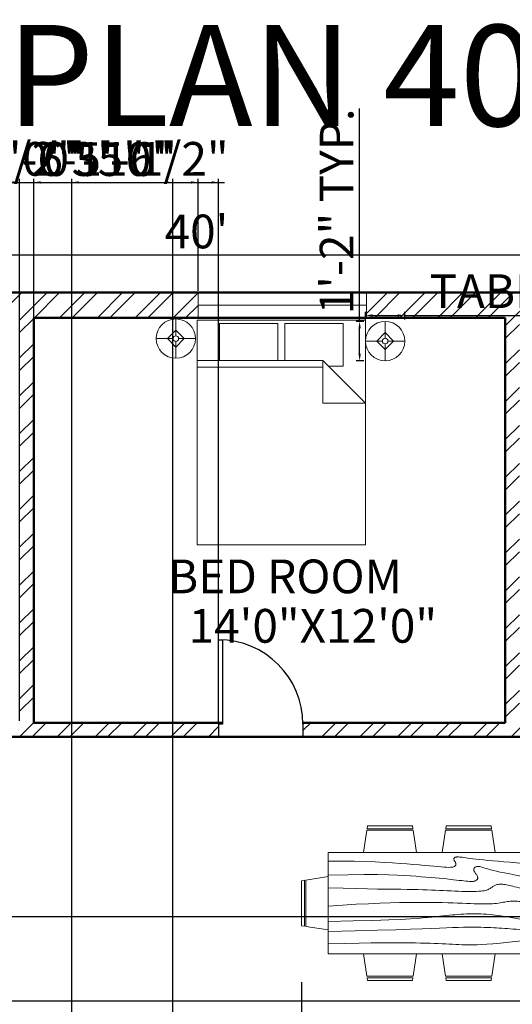
# Model space of a CAD drawing. Units: inches. Extents: x 1954 to 2815, y 1733 to 2371.
# Tile 3 of 4: x 2417 to 2592, y 2012 to 2362. Entities that reach past the tile are written whole.
import ezdxf

# ---------------------------------------------------------------- set-up
doc = ezdxf.new("R2010")
doc.units = ezdxf.units.IN
for name, color, linetype, lineweight in [('A-ANNO-DIMS', 2, 'Continuous', 18), ('A-ANNO-TEXT', 7, 'Continuous', 25), ('A-AREA-IDEN', 7, 'Continuous', 25), ('A-DOOR', 3, 'Continuous', 25), ('A-FURN', 8, 'Continuous', 18), ('A-GLAZ', 4, 'Continuous', 18), ('A-WALL', 7, 'Continuous', 50), ('A-WALL-PATT', 252, 'Continuous', 13)]:
    doc.layers.add(name, color=color, linetype=linetype, lineweight=lineweight)
doc.styles.get("Standard").update_dxf_attribs({"font": 'arial.ttf'})
doc.dimstyles.new('ISO-25', dxfattribs={"dimtxt": 12, "dimasz": 2.5, "dimexe": 1.25, "dimexo": 0.625, "dimtad": 1, "dimdec": 1, "dimlunit": 4, "dimtxsty": 'Standard', "dimcen": 2.5, "dimadec": 0, "dimazin": 0, "dimtfac": 1, "dimtdec": 1, "dimtmove": 0, "dimatfit": 3, "dimfxl": 1, "dimarcsym": 0})

# ---------------------------------------------------------------- blocks, each defined once
blk = doc.blocks.new('*U2')
for p, q in [((0, 0), (0, -6)), ((40, 0), (40, -6))]:
    blk.add_line(p, q)
blk.add_lwpolyline([(0, 0), (0, 40), (1.75, 40), (1.75, 0)], close=True)
blk.add_arc((0, 0), 40, 0, 90)
blk = doc.blocks.new('Bed - Queen')
for p, q in [((0, -80.00003), (0, 0)), ((0, 0), (59.99999, 0)), ((59.99999, 0), (59.99999, -80.00003)), ((7.99999, -1.2), (28.79998, -1.2)), ((7.99999, -14.4), (7.99999, -1.2)), ((28.79998, -1.2), (28.79998, -14.4)), ((31.19999, -1.2), (51.99999, -1.2)), ((31.19999, -14.4), (31.19999, -1.2)), ((51.99999, -1.2), (51.99999, -16.4)), ((0, -14.4), (44.8, -14.4)), ((44.8, -16.8), (0, -16.8)), ((59.99999, -29.6), (44.8, -14.4)), ((44.8, -14.4), (44.8, -29.6)), ((51.99999, -16.4), (46.79936, -16.4)), ((44.8, -29.6), (59.99999, -29.6)), ((59.99999, -80.00003), (0, -80.00003))]:
    blk.add_line(p, q)
blk = doc.blocks.new('Lamp - Table')
for p, q in [((0, 7), (0, 1)), ((-1, 0), (-7, 0)), ((0, 3), (-3, 0)), ((-3, 0), (0, -3)), ((3, 0), (0, 3)), ((0, -3), (3, 0)), ((1, 0), (7, 0)), ((0, -1), (0, -7))]:
    blk.add_line(p, q)
for radius in [7, 1]:
    blk.add_circle((0, 0), radius)
blk = doc.blocks.new('Dining Set - 36 x 72 in.')
for p, q in [((-22.2343, 26.00059), (-23.4847, 17.99762)), ((-22.2304, 26), (-5.7608, 26)), ((-22, 27.5), (-22.1562, 26.50042)), ((-5.8416, 26.5), (-22.1534, 26.5)), ((-22, 27.5), (-6, 27.5)), ((-5.8437, 26.49966), (-6, 27.5)), ((-4.5152, 17.99762), (-5.7655, 25.99926)), ((5.7657, 26.00059), (4.5153, 17.99762)), ((5.7696, 26), (22.2392, 26)), ((6, 27.5), (5.8438, 26.50042)), ((22.1584, 26.5), (5.8466, 26.5)), ((6, 27.5), (22, 27.5)), ((22.1563, 26.49966), (22, 27.5)), ((23.4848, 17.99762), (22.2345, 25.99926)), ((36, 18), (-36, 18)), ((-36, 18), (-36, -18)), ((36, -18), (36, 18)), ((-45.5, 8), (-44.5004, 8.15617)), ((-45.5, 8), (-45.5, -8)), ((-44.5, -8.15843), (-44.5, 8.15338)), ((-44.0006, 8.23428), (-35.9976, 9.48474)), ((-44, 8.23041), (-44, -8.23915)), ((44.0006, 8.23428), (35.9976, 9.48474)), ((44, 8.23041), (44, -8.23915)), ((44.5, -8.15843), (44.5, 8.15338)), ((45.5, 8), (44.5005, 8.15617)), ((45.5, 8), (45.5, -8)), ((-44.4997, -8.15631), (-45.5, -8)), ((-35.9976, -9.48476), (-43.9993, -8.2345)), ((35.9976, -9.48476), (43.9993, -8.2345)), ((44.4997, -8.15631), (45.5, -8)), ((-36, -18), (36, -18)), ((-22.2343, -26.0006), (-23.4847, -17.99762)), ((-4.5152, -17.99762), (-5.7655, -25.99928)), ((5.7657, -26.0006), (4.5153, -17.99762)), ((23.4848, -17.99762), (22.2345, -25.99928)), ((-22.2304, -26), (-5.7608, -26)), ((-22, -27.5), (-22.1562, -26.50044)), ((-5.8416, -26.5), (-22.1534, -26.5)), ((-22, -27.5), (-6, -27.5)), ((-5.8437, -26.49967), (-6, -27.5)), ((5.7696, -26), (22.2392, -26)), ((6, -27.5), (5.8438, -26.50044)), ((22.1584, -26.5), (5.8466, -26.5)), ((6, -27.5), (22, -27.5)), ((22.1563, -26.49967), (22, -27.5))]:
    blk.add_line(p, q)
for points in [[(-36, 15), (-31.1772, 14.97754), (-26.8079, 14.91406), (-22.8538, 14.81543), (-19.276, 14.6875), (-16.0362, 14.53613), (-13.0957, 14.36718), (-10.4159, 14.18652), (-7.9583, 14), (-5.6904, 13.81315), (-3.6035, 13.63021), (-1.6954, 13.45508), (0.0365, 13.29166), (1.5945, 13.14388), (2.9811, 13.01562), (4.1988, 12.9108), (5.25, 12.83333), (6.1393, 12.78613), (6.8802, 12.76823), (7.4883, 12.77767), (7.9792, 12.8125), (8.3685, 12.87077), (8.6719, 12.95052), (8.9049, 13.0498), (9.0833, 13.16666), (9.2205, 13.29899), (9.3216, 13.44401), (9.3895, 13.59879), (9.4271, 13.76041), (9.4373, 13.92594), (9.4232, 14.09245), (9.3875, 14.257), (9.3333, 14.41666), (9.2638, 14.56917), (9.1836, 14.71484), (9.0975, 14.85465), (9.0104, 14.98958), (8.9272, 15.1206), (8.8529, 15.2487), (8.7922, 15.37483), (8.75, 15.5), (8.7305, 15.62467), (8.7344, 15.74739), (8.7617, 15.86621), (8.8125, 15.97916), (8.8867, 16.08431), (8.9844, 16.17968), (9.1055, 16.26334), (9.25, 16.33333), (9.4189, 16.38802), (9.6172, 16.42708), (9.8506, 16.45052), (10.125, 16.45833), (10.4463, 16.45052), (10.8203, 16.42708), (11.2529, 16.38802), (11.75, 16.33333), (12.3184, 16.26318), (12.9694, 16.17838), (13.7151, 16.07991), (14.5677, 15.96875), (15.5395, 15.84586), (16.6426, 15.71224), (17.8893, 15.56884), (19.2917, 15.41666), (20.859, 15.25667), (22.5879, 15.08984), (24.4721, 14.91715), (26.5052, 14.73958), (28.6809, 14.5581), (30.9929, 14.3737), (33.4347, 14.18733), (36, 14)], [(-36, 10), (-28.9766, 10.14274), (-23.1725, 10.20442), (-18.4241, 10.19775), (-14.5677, 10.13541), (-11.4399, 10.03011), (-8.877, 9.89453), (-6.7154, 9.74137), (-4.7917, 9.58333), (-2.9698, 9.43082), (-1.2246, 9.28515), (0.4415, 9.14534), (2.026, 9.01041), (3.5266, 8.87939), (4.9408, 8.7513), (6.266, 8.62516), (7.5, 8.5), (8.6411, 8.37549), (9.6914, 8.2539), (10.6538, 8.13818), (11.5312, 8.03125), (12.3267, 7.93603), (13.043, 7.85547), (13.6831, 7.79248), (14.25, 7.75), (14.7471, 7.7303), (15.1797, 7.73307), (15.5537, 7.75732), (15.875, 7.80208), (16.1494, 7.86637), (16.3828, 7.94922), (16.5811, 8.04964), (16.75, 8.16666), (16.8944, 8.29915), (17.0143, 8.44531), (17.1089, 8.60319), (17.1771, 8.77083), (17.218, 8.94629), (17.2305, 9.1276), (17.2137, 9.31282), (17.1667, 9.5), (17.0895, 9.6875), (16.987, 9.875), (16.8649, 10.0625), (16.7292, 10.25), (16.5856, 10.4375), (16.4401, 10.625), (16.2985, 10.8125), (16.1667, 11), (16.05, 11.18733), (15.9518, 11.3737), (15.8752, 11.5581), (15.8229, 11.73958), (15.798, 11.91715), (15.8034, 12.08984), (15.842, 12.25667), (15.9167, 12.41666), (16.0295, 12.56836), (16.1784, 12.70833), (16.3605, 12.83268), (16.5729, 12.9375), (16.8127, 13.01888), (17.0768, 13.07291), (17.3625, 13.0957), (17.6667, 13.08333), (17.9894, 13.03312), (18.3418, 12.94726), (18.7382, 12.82918), (19.1927, 12.68229), (19.7195, 12.51001), (20.3327, 12.31575), (21.0465, 12.10294), (21.875, 11.875), (22.8357, 11.63354), (23.959, 11.37304), (25.2786, 11.08618), (26.8282, 10.76562), (28.6414, 10.40405), (30.752, 9.99414), (33.1936, 9.52856), (36, 9)], [(-36, 5.5), (-30.7157, 5.3348), (-26.069, 5.20963), (-21.9946, 5.11767), (-18.4271, 5.05208), (-15.3009, 5.00602), (-12.5508, 4.97265), (-10.1112, 4.94515), (-7.9167, 4.91666), (-5.909, 4.88167), (-4.0586, 4.83984), (-2.3429, 4.79215), (-0.7396, 4.73958), (0.7739, 4.6831), (2.22, 4.6237), (3.6213, 4.56233), (5, 4.5), (6.373, 4.43782), (7.7344, 4.3776), (9.0723, 4.32129), (10.375, 4.27083), (11.6309, 4.22819), (12.8281, 4.19531), (13.9551, 4.17415), (15, 4.16666), (15.954, 4.17448), (16.819, 4.19791), (17.6001, 4.23698), (18.3021, 4.29166), (18.9299, 4.36198), (19.4883, 4.44791), (19.9823, 4.54948), (20.4167, 4.66666), (20.7969, 4.79899), (21.1302, 4.94401), (21.4245, 5.09879), (21.6875, 5.26041), (21.9271, 5.42594), (22.1511, 5.59245), (22.3672, 5.757), (22.5834, 5.91666), (22.8065, 6.06868), (23.0404, 6.21093), (23.2879, 6.34147), (23.5521, 6.45833), (23.8358, 6.55957), (24.142, 6.64323), (24.4735, 6.70735), (24.8334, 6.75), (25.2235, 6.76969), (25.642, 6.76692), (26.0858, 6.74267), (26.5521, 6.69791), (27.0379, 6.63362), (27.5404, 6.55078), (28.0565, 6.45036), (28.5834, 6.33333), (29.1242, 6.19987), (29.7071, 6.04687), (30.3661, 5.87044), (31.1354, 5.66666), (32.0493, 5.43164), (33.142, 5.16146), (34.4475, 4.85221), (36, 4.5)], [(-36, -1), (-30.7915, -0.6591), (-26.0195, -0.38216), (-21.6519, -0.16284), (-17.6563, 0.00521), (-14.0005, 0.12833), (-10.6523, 0.21289), (-7.5796, 0.26522), (-4.75, 0.29166), (-2.134, 0.29793), (0.2878, 0.28711), (2.5317, 0.26163), (4.6146, 0.22396), (6.5529, 0.17651), (8.3633, 0.12174), (10.0623, 0.06209), (11.6667, 0), (13.1899, -0.06201), (14.6341, -0.1211), (15.9982, -0.17432), (17.2813, -0.21875), (18.4823, -0.25147), (19.6003, -0.26953), (20.6343, -0.27002), (21.5834, -0.25), (22.4481, -0.20768), (23.2357, -0.14584), (23.9549, -0.06836), (24.6146, 0.02083), (25.2235, 0.11784), (25.7904, 0.21875), (26.3241, 0.31966), (26.8334, 0.41666), (27.3265, 0.50618), (27.8099, 0.58593), (28.2894, 0.65397), (28.7709, 0.70833), (29.2601, 0.74707), (29.763, 0.76823), (30.2855, 0.76985), (30.8334, 0.75), (31.4088, 0.70784), (31.9994, 0.64713), (32.589, 0.57275), (33.1615, 0.48958), (33.7008, 0.4025), (34.1908, 0.3164), (34.6153, 0.23616), (34.9584, 0.16666), (35.2099, 0.11165), (35.3848, 0.07031), (35.504, 0.04069), (35.5886, 0.02083), (35.6594, 0.00879), (35.7377, 0.0026), (35.8442, 0.00032), (36, 0)], [(-36, -6.5), (-27.1843, -6.31267), (-20.084, -6.1263), (-14.469, -5.9419), (-10.1094, -5.76042), (-6.7752, -5.58285), (-4.2363, -5.41016), (-2.2629, -5.24333), (-0.625, -5.08334), (0.8708, -4.93099), (2.2715, -4.78646), (3.5872, -4.64974), (4.8281, -4.52084), (6.0046, -4.39974), (7.127, -4.28646), (8.2053, -4.18099), (9.25, -4.08334), (10.2705, -3.99382), (11.2734, -3.91407), (12.2647, -3.84603), (13.25, -3.79167), (14.2354, -3.75293), (15.2266, -3.73177), (16.2295, -3.73015), (17.25, -3.75), (18.2912, -3.79248), (19.3451, -3.85547), (20.4009, -3.93604), (21.4479, -4.03125), (22.4754, -4.13819), (23.4727, -4.25391), (24.4289, -4.37549), (25.3334, -4.5), (26.1785, -4.62492), (26.9694, -4.74935), (27.7145, -4.87281), (28.4219, -4.99479), (29.1, -5.11483), (29.7572, -5.23242), (30.4016, -5.34709), (31.0417, -5.45834), (31.6837, -5.56437), (32.3262, -5.65821), (32.9658, -5.73153), (33.599, -5.77604), (34.2224, -5.78345), (34.8327, -5.74545), (35.4264, -5.65373), (36, -5.5)], [(-36, -10), (-26.4022, -9.81299), (-18.4675, -9.62891), (-11.9839, -9.45069), (-6.7396, -9.28125), (-2.5226, -9.12354), (0.8789, -8.98047), (3.6769, -8.85498), (6.0833, -8.75), (8.2767, -8.66765), (10.3021, -8.60677), (12.1712, -8.56543), (13.8958, -8.54167), (15.4876, -8.53353), (16.9583, -8.53907), (18.3197, -8.55632), (19.5834, -8.58334), (20.7616, -8.61841), (21.8685, -8.66081), (22.9188, -8.71004), (23.9271, -8.76563), (24.9081, -8.82707), (25.8763, -8.89388), (26.8465, -8.96558), (27.8334, -9.04167), (28.8474, -9.12118), (29.8828, -9.20117), (30.93, -9.27824), (31.9792, -9.34896), (33.0205, -9.40991), (34.0443, -9.45768), (35.0407, -9.48885), (36, -9.5)], [(-36, -14.5), (-30.0881, -14.33513), (-25.0332, -14.21224), (-20.7312, -14.12647), (-17.0781, -14.07292), (-13.97, -14.04671), (-11.3027, -14.04297), (-8.9724, -14.05681), (-6.875, -14.08334), (-4.9224, -14.11833), (-3.0905, -14.16016), (-1.3709, -14.20785), (0.2448, -14.26042), (1.7647, -14.3169), (3.1973, -14.3763), (4.5507, -14.43767), (5.8333, -14.5), (7.0554, -14.5621), (8.235, -14.62175), (9.3922, -14.67652), (10.5469, -14.72396), (11.7192, -14.76164), (12.929, -14.78711), (14.1965, -14.79794), (15.5417, -14.79167), (16.9933, -14.76424), (18.6152, -14.70508), (20.4804, -14.60197), (22.6615, -14.44271), (25.2312, -14.21509), (28.2624, -13.9069), (31.8277, -13.50594), (36, -13)]]:
    blk.add_lwpolyline(points)
blk = doc.blocks.new('*D10')
at = {"layer": 'A-ANNO-DIMS', "color": 0, "lineweight": -2, "transparency": 16777216}
for p, q in [((2239.88, 2265.61), (2239.88, 2279.68)), ((2242.38, 2278.43), (2717.38, 2278.43)), ((2719.88, 2265.61), (2719.88, 2279.68))]:
    blk.add_line(p, q, dxfattribs=at)
at = {"layer": 'A-ANNO-DIMS', "color": 0, "transparency": 16777216}
for points in [[(2242.38, 2278.85), (2242.38, 2278.01), (2239.88, 2278.43)], [(2717.38, 2278.85), (2717.38, 2278.01), (2719.88, 2278.43)]]:
    blk.add_solid(points, dxfattribs=at)
at = {"layer": 'Defpoints', "color": 0, "transparency": 16777216}
for p in [(2719.88, 2278.43), (2239.88, 2264.98), (2719.88, 2264.98)]:
    blk.add_point(p, dxfattribs=at)
at = {"layer": 'A-ANNO-DIMS', "color": 0, "transparency": 16777216, "insert": (2479.88, 2285.18), "char_height": 12, "attachment_point": 5}
blk.add_mtext("40'", dxfattribs=at)
blk = doc.blocks.new('*D16')
at = {"layer": 'A-ANNO-DIMS', "color": 0, "lineweight": -2, "transparency": 16777216}
for p, q in [((2540.09, 2255.38), (2540.09, 2258.1)), ((2542.59, 2256.85), (2551.59, 2256.85)), ((2554.09, 2255.38), (2554.09, 2258.1)), ((2554.09, 2256.85), (2757.06, 2256.85))]:
    blk.add_line(p, q, dxfattribs=at)
at = {"layer": 'A-ANNO-DIMS', "color": 0, "transparency": 16777216}
for points in [[(2542.59, 2257.27), (2542.59, 2256.44), (2540.09, 2256.85)], [(2551.59, 2257.27), (2551.59, 2256.44), (2554.09, 2256.85)]]:
    blk.add_solid(points, dxfattribs=at)
at = {"layer": 'Defpoints', "color": 0, "transparency": 16777216}
for p in [(2554.09, 2256.85), (2540.09, 2254.75), (2554.09, 2254.75)]:
    blk.add_point(p, dxfattribs=at)
at = {"layer": 'A-ANNO-DIMS', "color": 0, "transparency": 16777216, "insert": (2656.83, 2263.94), "char_height": 12, "attachment_point": 5}
blk.add_mtext('TABLE LAMP Ø 1\'-2" TYP.', dxfattribs=at)
blk = doc.blocks.new('*D17')
at = {"layer": 'A-ANNO-DIMS', "color": 0, "lineweight": -2, "transparency": 16777216}
for p, q in [((2537.99, 2254.75), (2537.99, 2330.52)), ((2539.47, 2254.75), (2536.74, 2254.75)), ((2537.99, 2243.25), (2537.99, 2252.25)), ((2539.47, 2240.75), (2536.74, 2240.75))]:
    blk.add_line(p, q, dxfattribs=at)
at = {"layer": 'A-ANNO-DIMS', "color": 0, "transparency": 16777216}
for points in [[(2537.57, 2252.25), (2538.41, 2252.25), (2537.99, 2254.75)], [(2537.57, 2243.25), (2538.41, 2243.25), (2537.99, 2240.75)]]:
    blk.add_solid(points, dxfattribs=at)
at = {"layer": 'Defpoints', "color": 0, "transparency": 16777216}
for p in [(2537.99, 2254.75), (2540.09, 2254.75), (2540.09, 2240.75)]:
    blk.add_point(p, dxfattribs=at)
at = {"layer": 'A-ANNO-DIMS', "color": 0, "transparency": 16777216, "insert": (2531.34, 2293.89), "char_height": 12, "attachment_point": 5, "rotation": 90}
blk.add_mtext('1\'-2" TYP.', dxfattribs=at)
blk = doc.blocks.new('*D24')
at = {"layer": 'A-ANNO-DIMS', "color": 0, "lineweight": -2, "transparency": 16777216}
for p, q in [((2517.32, 2019.64), (2517.32, 2005.36)), ((2608.32, 2019.64), (2608.32, 2005.36)), ((2519.82, 2006.61), (2605.82, 2006.61)), ((2608.32, 2006.61), (2743.97, 2006.61))]:
    blk.add_line(p, q, dxfattribs=at)
at = {"layer": 'A-ANNO-DIMS', "color": 0, "transparency": 16777216}
for points in [[(2519.82, 2007.03), (2519.82, 2006.2), (2517.32, 2006.61)], [(2605.82, 2007.03), (2605.82, 2006.2), (2608.32, 2006.61)]]:
    blk.add_solid(points, dxfattribs=at)
at = {"layer": 'Defpoints', "color": 0, "transparency": 16777216}
for p in [(2517.32, 2020.26), (2608.32, 2020.26), (2608.32, 2006.61)]:
    blk.add_point(p, dxfattribs=at)
at = {"layer": 'A-ANNO-DIMS', "color": 0, "transparency": 16777216, "insert": (2677.39, 2013.44), "char_height": 12, "attachment_point": 5}
blk.add_mtext('DINING SET 7\'-7"', dxfattribs=at)
blk = doc.blocks.new('*D37')
at = {"layer": 'A-ANNO-DIMS', "color": 0, "lineweight": -2, "transparency": 16777216}
for p, q in [((2416.88, 2256.61), (2416.88, 2305.43)), ((2421.88, 2256.61), (2421.88, 2305.43)), ((2414.38, 2304.18), (2411.88, 2304.18)), ((2416.88, 2304.18), (2421.88, 2304.18)), ((2424.38, 2304.18), (2460.03, 2304.18))]:
    blk.add_line(p, q, dxfattribs=at)
at = {"layer": 'A-ANNO-DIMS', "color": 0, "transparency": 16777216}
for points in [[(2414.38, 2304.6), (2414.38, 2303.77), (2416.88, 2304.18)], [(2424.38, 2304.6), (2424.38, 2303.77), (2421.88, 2304.18)]]:
    blk.add_solid(points, dxfattribs=at)
at = {"layer": 'Defpoints', "color": 0, "transparency": 16777216}
for p in [(2421.88, 2304.18), (2416.88, 2255.98), (2421.88, 2255.98)]:
    blk.add_point(p, dxfattribs=at)
at = {"layer": 'A-ANNO-DIMS', "color": 0, "transparency": 16777216, "insert": (2443.46, 2310.93), "char_height": 12, "attachment_point": 5}
blk.add_mtext('0\'-5"', dxfattribs=at)
blk = doc.blocks.new('*D39')
at = {"layer": 'A-ANNO-DIMS', "color": 0, "lineweight": -2, "transparency": 16777216}
for p, q in [((2354.46, 2265.61), (2354.46, 2305.43)), ((2480.43, 2265.61), (2480.43, 2305.43)), ((2356.96, 2304.18), (2477.93, 2304.18))]:
    blk.add_line(p, q, dxfattribs=at)
at = {"layer": 'A-ANNO-DIMS', "color": 0, "transparency": 16777216}
for points in [[(2356.96, 2304.6), (2356.96, 2303.77), (2354.46, 2304.18)], [(2477.93, 2304.6), (2477.93, 2303.77), (2480.43, 2304.18)]]:
    blk.add_solid(points, dxfattribs=at)
at = {"layer": 'Defpoints', "color": 0, "transparency": 16777216}
for p in [(2480.43, 2304.18), (2354.46, 2264.98), (2480.43, 2264.98)]:
    blk.add_point(p, dxfattribs=at)
at = {"layer": 'A-ANNO-DIMS', "color": 0, "transparency": 16777216, "insert": (2417.44, 2310.93), "char_height": 12, "attachment_point": 5}
blk.add_mtext('10\'-6"', dxfattribs=at)
blk = doc.blocks.new('*D47')
at = {"layer": 'A-ANNO-DIMS', "color": 0, "lineweight": -2, "transparency": 16777216}
for p, q in [((2375.36, 2106.36), (2375.36, 1768.53)), ((2405.36, 2106.36), (2405.36, 1768.53)), ((2377.86, 1769.78), (2402.86, 1769.78)), ((2405.36, 1769.78), (2441.21, 1769.78))]:
    blk.add_line(p, q, dxfattribs=at)
at = {"layer": 'A-ANNO-DIMS', "color": 0, "transparency": 16777216}
for points in [[(2377.86, 1770.2), (2377.86, 1769.37), (2375.36, 1769.78)], [(2402.86, 1770.2), (2402.86, 1769.37), (2405.36, 1769.78)]]:
    blk.add_solid(points, dxfattribs=at)
at = {"layer": 'Defpoints', "color": 0, "transparency": 16777216}
for p in [(2375.36, 2106.98), (2405.36, 2106.98), (2405.36, 1769.78)]:
    blk.add_point(p, dxfattribs=at)
at = {"layer": 'A-ANNO-DIMS', "color": 0, "transparency": 16777216, "insert": (2424.53, 1776.53), "char_height": 12, "attachment_point": 5}
blk.add_mtext('2\'-6"', dxfattribs=at)
blk = doc.blocks.new('*D48')
at = {"layer": 'A-ANNO-DIMS', "color": 0, "lineweight": -2, "transparency": 16777216}
for p, q in [((2405.35, 2112.61), (2405.35, 2305.43)), ((2416.88, 2112.61), (2416.88, 2305.43)), ((2407.85, 2304.18), (2414.38, 2304.18)), ((2416.88, 2304.18), (2489.82, 2304.18))]:
    blk.add_line(p, q, dxfattribs=at)
at = {"layer": 'A-ANNO-DIMS', "color": 0, "transparency": 16777216}
for points in [[(2407.85, 2304.6), (2407.85, 2303.77), (2405.35, 2304.18)], [(2414.38, 2304.6), (2414.38, 2303.77), (2416.88, 2304.18)]]:
    blk.add_solid(points, dxfattribs=at)
at = {"layer": 'Defpoints', "color": 0, "transparency": 16777216}
for p in [(2416.88, 2304.18), (2405.35, 2111.98), (2416.88, 2111.98)]:
    blk.add_point(p, dxfattribs=at)
at = {"layer": 'A-ANNO-DIMS', "color": 0, "transparency": 16777216, "insert": (2454.6, 2311.01), "char_height": 12, "attachment_point": 5}
blk.add_mtext('0\'-11 1/2"', dxfattribs=at)
blk = doc.blocks.new('*D49')
at = {"layer": 'A-ANNO-DIMS', "color": 0, "lineweight": -2, "transparency": 16777216}
for p, q in [((2421.88, 2112.61), (2421.88, 2305.43)), ((2487.77, 2112.11), (2487.77, 2305.43)), ((2424.38, 2304.18), (2485.27, 2304.18))]:
    blk.add_line(p, q, dxfattribs=at)
at = {"layer": 'A-ANNO-DIMS', "color": 0, "transparency": 16777216}
for points in [[(2424.38, 2304.6), (2424.38, 2303.77), (2421.88, 2304.18)], [(2485.27, 2304.6), (2485.27, 2303.77), (2487.77, 2304.18)]]:
    blk.add_solid(points, dxfattribs=at)
at = {"layer": 'Defpoints', "color": 0, "transparency": 16777216}
for p in [(2487.77, 2304.18), (2421.88, 2111.98), (2487.77, 2111.48)]:
    blk.add_point(p, dxfattribs=at)
at = {"layer": 'A-ANNO-DIMS', "color": 0, "transparency": 16777216, "insert": (2454.83, 2310.93), "char_height": 12, "attachment_point": 5}
blk.add_mtext('5\'-6"', dxfattribs=at)
blk = doc.blocks.new('*D52')
at = {"layer": 'A-ANNO-DIMS', "color": 0, "lineweight": -2, "transparency": 16777216}
for p, q in [((2759.08, 2043), (2759.08, 2078.85)), ((2344.56, 2043), (2760.33, 2043)), ((2759.08, 2015.5), (2759.08, 2040.5)), ((2344.56, 2013), (2760.33, 2013))]:
    blk.add_line(p, q, dxfattribs=at)
at = {"layer": 'A-ANNO-DIMS', "color": 0, "transparency": 16777216}
for points in [[(2758.67, 2040.5), (2759.5, 2040.5), (2759.08, 2043)], [(2758.67, 2015.5), (2759.5, 2015.5), (2759.08, 2013)]]:
    blk.add_solid(points, dxfattribs=at)
at = {"layer": 'Defpoints', "color": 0, "transparency": 16777216}
for p in [(2343.94, 2043), (2759.08, 2043), (2343.94, 2013)]:
    blk.add_point(p, dxfattribs=at)
at = {"layer": 'A-ANNO-DIMS', "color": 0, "transparency": 16777216, "insert": (2752.33, 2062.18), "char_height": 12, "attachment_point": 5, "rotation": 90}
blk.add_mtext('2\'-6"', dxfattribs=at)
blk = doc.blocks.new('*D53')
at = {"layer": 'A-ANNO-DIMS', "color": 0, "lineweight": -2, "transparency": 16777216}
for p, q in [((2435.43, 1943.61), (2435.43, 2305.43)), ((2471.49, 1943.61), (2471.49, 2305.43)), ((2437.93, 2304.18), (2468.99, 2304.18))]:
    blk.add_line(p, q, dxfattribs=at)
at = {"layer": 'A-ANNO-DIMS', "color": 0, "transparency": 16777216}
for points in [[(2437.93, 2304.6), (2437.93, 2303.77), (2435.43, 2304.18)], [(2468.99, 2304.6), (2468.99, 2303.77), (2471.49, 2304.18)]]:
    blk.add_solid(points, dxfattribs=at)
at = {"layer": 'Defpoints', "color": 0, "transparency": 16777216}
for p in [(2471.49, 2304.18), (2435.43, 1942.98), (2471.49, 1942.98)]:
    blk.add_point(p, dxfattribs=at)
at = {"layer": 'A-ANNO-DIMS', "color": 0, "transparency": 16777216, "insert": (2453.46, 2310.94), "char_height": 12, "attachment_point": 5}
blk.add_mtext('3\'-0"', dxfattribs=at)
blk = doc.blocks.new('*D55')
at = {"layer": 'A-ANNO-DIMS', "color": 0, "lineweight": -2, "transparency": 16777216}
for p, q in [((2343.88, 1989.61), (2343.88, 2305.43)), ((2372.59, 1990.74), (2372.59, 2305.43)), ((2346.38, 2304.18), (2370.09, 2304.18)), ((2372.59, 2304.18), (2436.4, 2304.18))]:
    blk.add_line(p, q, dxfattribs=at)
at = {"layer": 'A-ANNO-DIMS', "color": 0, "transparency": 16777216}
for points in [[(2346.38, 2304.6), (2346.38, 2303.77), (2343.88, 2304.18)], [(2370.09, 2304.6), (2370.09, 2303.77), (2372.59, 2304.18)]]:
    blk.add_solid(points, dxfattribs=at)
at = {"layer": 'Defpoints', "color": 0, "transparency": 16777216}
for p in [(2372.59, 2304.18), (2372.59, 1990.12), (2343.88, 1988.98)]:
    blk.add_point(p, dxfattribs=at)
at = {"layer": 'A-ANNO-DIMS', "color": 0, "transparency": 16777216, "insert": (2405.75, 2311.01), "char_height": 12, "attachment_point": 5}
blk.add_mtext('2\'-4 1/2"', dxfattribs=at)

msp = doc.modelspace()

# ---------------------------------------------------------------- hatches: boundary and pattern name
at = {"layer": 'A-WALL-PATT'}
h = msp.add_hatch(dxfattribs=at)
h.set_pattern_fill('ANSI32', color=256)
h.paths.add_polyline_path([(2480.43, 2264.98), (2354.46, 2264.98), (2354.46, 2255.98), (2416.88, 2255.98), (2416.88, 2111.98), (2405.35, 2111.98, -0.004167), (2405.36, 2111.48), (2405.36, 2106.98), (2487.77, 2106.98), (2487.77, 2111.48), (2487.77, 2111.98), (2421.88, 2111.98), (2421.88, 2255.98), (2480.43, 2255.98)])
h.paths.add_polyline_path([(2719.88, 2264.98), (2540.43, 2264.98), (2540.43, 2255.98), (2589.88, 2255.98), (2589.88, 2111.98), (2517.77, 2111.98, -0.004167), (2517.77, 2111.48), (2517.77, 2106.98), (2631.3, 2106.98), (2631.3, 2111.98), (2594.88, 2111.98), (2594.88, 2255.98), (2710.88, 2255.98), (2710.88, 2213), (2719.88, 2213)])

# ---------------------------------------------------------------- linework, layer by layer
at = {"layer": 'A-GLAZ'}
msp.add_line((2480.43, 2260.48), (2540.43, 2260.48), dxfattribs=at)
msp.add_lwpolyline([(2480.43, 2264.98), (2540.43, 2264.98), (2540.43, 2255.98), (2480.43, 2255.98)], close=True, dxfattribs=at)
at = {"layer": 'A-WALL'}
for p, q in [((2239.88, 2264.98), (2719.88, 2264.98)), ((2421.88, 2255.98), (2589.88, 2255.98)), ((2421.88, 2111.98), (2421.88, 2255.98)), ((2589.88, 2111.98), (2589.88, 2255.98)), ((2421.88, 2111.98), (2489.08, 2111.98)), ((2517.77, 2111.98), (2589.88, 2111.98)), ((2343.88, 2106.98), (2631.3, 2106.98))]:
    msp.add_line(p, q, dxfattribs=at)

# ---------------------------------------------------------------- block references
at = {"layer": 'A-DOOR', "xscale": 0.75, "yscale": 0.75, "zscale": 0.75}
msp.add_blockref('*U2', (2487.77, 2111.48), dxfattribs=at)
at = {"layer": 'A-FURN'}
for name, p in [('Lamp - Table', (2472.52, 2248.61)), ('Bed - Queen', (2480.09, 2255.23)), ('Lamp - Table', (2547.09, 2247.75)), ('Dining Set - 36 x 72 in.', (2562.82, 2047.76))]:
    msp.add_blockref(name, p, dxfattribs=at)

# ---------------------------------------------------------------- texts
at = {"layer": 'A-ANNO-TEXT'}
msp.add_text('3BHK HOUSE PLAN 40\'0"X35\'0"', height=36, dxfattribs=at).set_placement((2097.45, 2324.21))
at = {"layer": 'A-AREA-IDEN'}
for s, p in [('BED ROOM', (2469.73, 2158.03)), ('14\'0"X12\'0"', (2477.07, 2140.44))]:
    msp.add_text(s, height=12, dxfattribs=at).set_placement(p)

# ---------------------------------------------------------------- dimensions: what is measured, and where the dimension line sits
at = {"layer": 'A-ANNO-DIMS'}
dim = msp.add_linear_dim(base=(2537.99, 2254.75), p1=(2540.09, 2240.75), p2=(2540.09, 2254.75), angle=90, text='<> TYP.', dimstyle='ISO-25', override={"dimdec": 1, "dimlfac": 1, "dimrnd": 0, "dimzin": 1, "dimdsep": 46, "dimlunit": 4, "dimfrac": 2}, dxfattribs=at)
dim.commit()
dim.dimension.update_dxf_attribs({"geometry": '*D17', "text_midpoint": (2531.34, 2293.89)})
for base, p1, p2, override, picture, middle in [((2372.59, 2304.18), (2343.88, 1988.98), (2372.59, 1990.12), {"dimdec": 1, "dimlfac": 1, "dimrnd": 0, "dimzin": 1, "dimdsep": 46, "dimlunit": 4, "dimfrac": 2}, '*D55', (2405.75, 2311.01)), ((2416.88, 2304.18), (2405.35, 2111.98), (2416.88, 2111.98), {"dimdec": 1, "dimlfac": 1, "dimrnd": 0, "dimzin": 1, "dimdsep": 46, "dimlunit": 4, "dimfrac": 2}, '*D48', (2454.6, 2311.01)), ((2480.43, 2304.18), (2354.46, 2264.98), (2480.43, 2264.98), {"dimdec": 1, "dimlfac": 1, "dimrnd": 0, "dimzin": 1, "dimdsep": 46, "dimlunit": 4, "dimfrac": 2}, '*D39', (2417.44, 2310.93)), ((2421.88, 2304.18), (2416.88, 2255.98), (2421.88, 2255.98), {"dimdec": 1, "dimlfac": 1, "dimrnd": 0, "dimzin": 1, "dimdsep": 46, "dimlunit": 4, "dimfrac": 2}, '*D37', (2443.46, 2310.93)), ((2487.77, 2304.18), (2421.88, 2111.98), (2487.77, 2111.48), {"dimdec": 1, "dimlfac": 1, "dimrnd": 0, "dimzin": 1, "dimdsep": 46, "dimlunit": 4, "dimfrac": 2}, '*D49', (2454.83, 2310.93)), ((2471.49, 2304.18), (2435.43, 1942.98), (2471.49, 1942.98), {"dimdec": 1, "dimlfac": 1, "dimrnd": 0, "dimzin": 1, "dimdsep": 46, "dimlunit": 4, "dimfrac": 2}, '*D53', (2453.46, 2310.94)), ((2719.88, 2278.43), (2239.88, 2264.98), (2719.88, 2264.98), {"dimclrd": 0, "dimclre": 0, "dimclrt": 0}, '*D10', (2479.88, 2285.18)), ((2405.36, 1769.78), (2375.36, 2106.98), (2405.36, 2106.98), {"dimdec": 1, "dimlfac": 1, "dimrnd": 0, "dimzin": 1, "dimdsep": 46, "dimlunit": 4, "dimfrac": 2}, '*D47', (2424.53, 1776.53))]:
    dim = msp.add_linear_dim(base=base, p1=p1, p2=p2, dimstyle='ISO-25', override=override, dxfattribs=at)
    dim.commit()
    dim.dimension.update_dxf_attribs({"geometry": picture, "text_midpoint": middle})
for base, p1, p2, text, picture, middle in [((2554.09, 2256.85), (2540.09, 2254.75), (2554.09, 2254.75), 'TABLE LAMP Ø <> TYP.', '*D16', (2656.83, 2263.94)), ((2608.32, 2006.61), (2517.32, 2020.26), (2608.32, 2020.26), 'DINING SET <>', '*D24', (2677.39, 2013.44))]:
    dim = msp.add_linear_dim(base=base, p1=p1, p2=p2, text=text, dimstyle='ISO-25', override={"dimdec": 1, "dimlfac": 1, "dimrnd": 0, "dimzin": 1, "dimdsep": 46, "dimlunit": 4, "dimfrac": 2}, dxfattribs=at)
    dim.commit()
    dim.dimension.update_dxf_attribs({"geometry": picture, "text_midpoint": middle})
dim = msp.add_linear_dim(base=(2759.08, 2043), p1=(2343.94, 2013), p2=(2343.94, 2043), angle=90, dimstyle='ISO-25', override={"dimdec": 1, "dimlfac": 1, "dimrnd": 0, "dimzin": 1, "dimdsep": 46, "dimlunit": 4, "dimfrac": 2}, dxfattribs=at)
dim.commit()
dim.dimension.update_dxf_attribs({"geometry": '*D52', "text_midpoint": (2752.33, 2062.18)})

doc.saveas('drawing.dxf')
